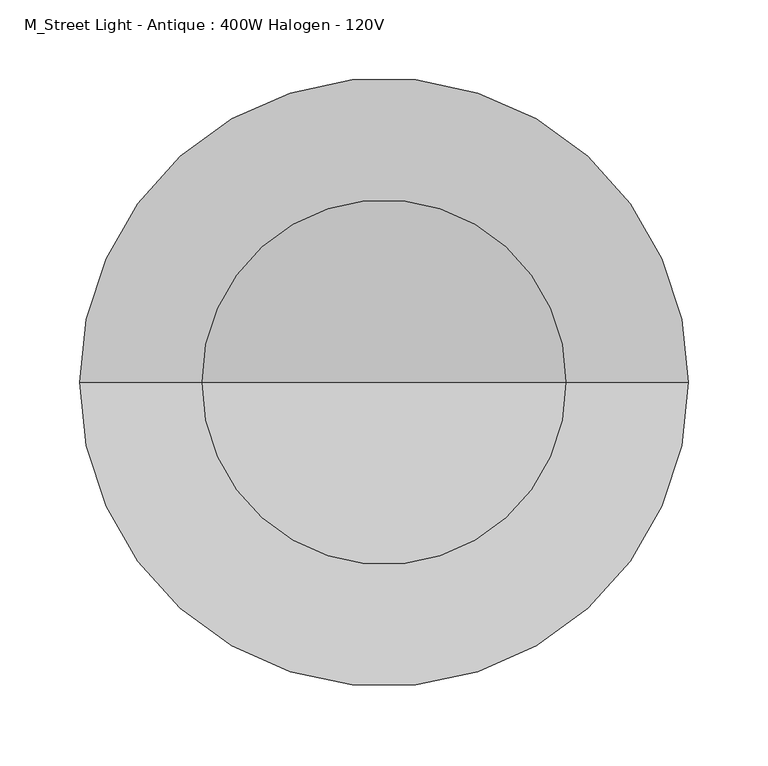
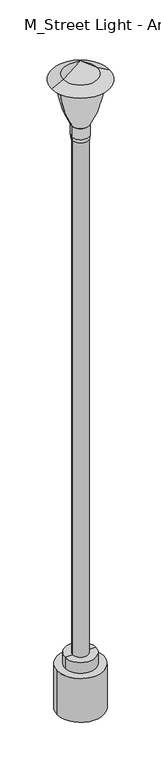
"""IFC4 building model written with IfcOpenShell, lengths in millimetres: light fixture geometry, M_Street Light - Antique : 400W Halogen - 120V."""

from ifc_helpers import new_model, si_unit, point, frame, origin, origin_with_axes, origin_2d, place, context, project, spatial, polyline, circle_curve, ellipse_curve, trimmed, segment, composite_curve, outline, extrude, source, transform, mapped, element, save
from ifc_brep_helpers import plane_surface, cylinder_surface, revolved_surface, advanced_brep


def m_street_light_antique_400w_halogen_120v_ac89fb25(model_context):
    return source(origin(), model_context, "Body", "SolidModel", [
        extrude(outline(composite_curve([segment(trimmed(circle_curve(origin_2d(), 152.4), [point((-152.4, 0.0))], [point((152.4, 0.0))], False, "CARTESIAN"), True, "CONTINUOUS"), segment(trimmed(circle_curve(origin_2d(), 152.4), [point((152.4, 0.0))], [point((-152.4, 0.0))], False, "CARTESIAN"), True, "CONTINUOUS")], self_intersect=False)), origin_with_axes(), (0.0, 0.0, 1.0), 304.8),
        advanced_brep(
        [(190.5, 0.0, 4373.0), (-190.5, 0.0, 4373.0), (-114.3, 0.0, 4411.1), (114.3, 0.0, 4411.1), (114.3, 0.0, 4373.0), (-114.3, 0.0, 4373.0), (114.3, 0.0, 4381.73125), (-114.3, 0.0, 4381.73125), (144.6394367, 0.0, 4381.73125), (-144.6394367, 0.0, 4381.73125), (107.4535144, 0.0, 4400.3242111), (-107.4535144, 0.0, 4400.3242111), (0.0, 0.0, 4485.1715369), (0.0, 0.0, 4500.0)],
        [
            (0, 1, circle_curve(frame((0.0, 0.0, 4373.0), z_axis=(0.0, 0.0, 1.0), x_axis=(-1.0, 0.0, 0.0)), 190.5)),
            (1, 2),
            (2, 3, circle_curve(frame((0.0, 0.0, 4411.1), z_axis=(0.0, 0.0, -1.0), x_axis=(-1.0, 0.0, 0.0)), 114.3)),
            (3, 0),
            (1, 0, circle_curve(frame((0.0, 0.0, 4373.0), z_axis=(0.0, 0.0, 1.0), x_axis=(-1.0, 0.0, 0.0)), 190.5)),
            (3, 2, circle_curve(frame((0.0, 0.0, 4411.1), z_axis=(0.0, 0.0, -1.0), x_axis=(-1.0, 0.0, 0.0)), 114.3)),
            (4, 5, circle_curve(frame((0.0, 0.0, 4373.0), z_axis=(0.0, 0.0, 1.0), x_axis=(-1.0, 0.0, 0.0)), 114.3)),
            (5, 1),
            (0, 4),
            (5, 4, circle_curve(frame((0.0, 0.0, 4373.0), z_axis=(0.0, 0.0, 1.0), x_axis=(-1.0, 0.0, 0.0)), 114.3)),
            (6, 7, circle_curve(frame((0.0, 0.0, 4381.73125), z_axis=(0.0, 0.0, 1.0), x_axis=(-1.0, 0.0, 0.0)), 114.3)),
            (7, 5),
            (4, 6),
            (7, 6, circle_curve(frame((0.0, 0.0, 4381.73125), z_axis=(0.0, 0.0, 1.0), x_axis=(-1.0, 0.0, 0.0)), 114.3)),
            (8, 9, circle_curve(frame((0.0, 0.0, 4381.73125), z_axis=(0.0, 0.0, 1.0), x_axis=(-1.0, 0.0, 0.0)), 144.6394367)),
            (9, 7),
            (6, 8),
            (9, 8, circle_curve(frame((0.0, 0.0, 4381.73125), z_axis=(0.0, 0.0, 1.0), x_axis=(-1.0, 0.0, 0.0)), 144.6394367)),
            (10, 11, circle_curve(frame((0.0, 0.0, 4400.3242111), z_axis=(0.0, 0.0, 1.0), x_axis=(-1.0, 0.0, 0.0)), 107.4535144)),
            (11, 9),
            (8, 10),
            (11, 10, circle_curve(frame((0.0, 0.0, 4400.3242111), z_axis=(0.0, 0.0, 1.0), x_axis=(-1.0, 0.0, 0.0)), 107.4535144)),
            (12, 11),
            (10, 12),
            (2, 13),
            (13, 3),
        ],
        [
            revolved_surface(polyline([(-114.3, 0.0, 4411.1), (-190.5, 0.0, 4373.0)]), (0.0, 0.0, 4754.0), (0.0, 0.0, -1.0)),
            plane_surface(frame((0.0, 0.0, 4373.0), z_axis=(0.0, 0.0, -1.0), x_axis=(-1.0, 0.0, 0.0))),
            revolved_surface(polyline([(-114.3, 0.0, 4373.0), (-114.3, 0.0, 4381.73125)]), (0.0, 0.0, 4754.0), (0.0, 0.0, -1.0)),
            plane_surface(frame((0.0, 0.0, 4381.73125), z_axis=(0.0, 0.0, 1.0), x_axis=(-1.0, 0.0, 0.0))),
            revolved_surface(polyline([(-144.6394367, 0.0, 4381.73125), (-107.4535144, 0.0, 4400.3242111)]), (0.0, 0.0, 4754.0), (0.0, 0.0, -1.0)),
            revolved_surface(polyline([(-107.4535144, 0.0, 4400.3242111), (0.0, 0.0, 4485.1715369)]), (0.0, 0.0, 4754.0), (0.0, 0.0, -1.0)),
            revolved_surface(polyline([(0.0, 0.0, 4500.0), (-114.3, 0.0, 4411.1)]), (0.0, 0.0, 4754.0), (0.0, 0.0, -1.0)),
        ],
        [
            (0, [[1, 2, 3, 4]]),
            (0, [[5, -4, 6, -2]]),
            (1, [[7, 8, -1, 9]]),
            (1, [[10, -9, -5, -8]]),
            (2, [[11, 12, -7, 13]]),
            (2, [[14, -13, -10, -12]]),
            (3, [[15, 16, -11, 17]]),
            (3, [[18, -17, -14, -16]]),
            (4, [[19, 20, -15, 21]]),
            (4, [[22, -21, -18, -20]]),
            (5, [[23, -19, 24]]),
            (5, [[-24, -22, -23]]),
            (6, [[-3, 25, 26]]),
            (6, [[-6, -26, -25]]),
        ],
    ),
        advanced_brep(
        [(53.975, 0.0, 3992.0), (-53.975, 0.0, 3992.0), (-57.3982763, 0.0, 3992.0), (57.3982763, 0.0, 3992.0), (53.975, 0.0, 3966.6), (-53.975, 0.0, 3966.6), (12.7, 0.0, 3966.6), (-12.7, 0.0, 3966.6), (12.7, 0.0, 3992.0), (-12.7, 0.0, 3992.0), (31.9982763, 0.0, 3992.0), (-31.9982763, 0.0, 3992.0), (31.9982763, 0.0, 4068.2), (-31.9982763, 0.0, 4068.2), (57.3982763, 0.0, 4068.2), (-57.3982763, 0.0, 4068.2)],
        [
            (0, 1, circle_curve(frame((0.0, 0.0, 3992.0), z_axis=(0.0, 0.0, 1.0), x_axis=(-1.0, 0.0, 0.0)), 53.975)),
            (1, 2),
            (2, 3, circle_curve(frame((0.0, 0.0, 3992.0), z_axis=(0.0, 0.0, -1.0), x_axis=(-1.0, 0.0, 0.0)), 57.3982763)),
            (3, 0),
            (1, 0, circle_curve(frame((0.0, 0.0, 3992.0), z_axis=(0.0, 0.0, 1.0), x_axis=(-1.0, 0.0, 0.0)), 53.975)),
            (3, 2, circle_curve(frame((0.0, 0.0, 3992.0), z_axis=(0.0, 0.0, -1.0), x_axis=(-1.0, 0.0, 0.0)), 57.3982763)),
            (4, 5, circle_curve(frame((0.0, 0.0, 3966.6), z_axis=(0.0, 0.0, 1.0), x_axis=(-1.0, 0.0, 0.0)), 53.975)),
            (5, 1),
            (0, 4),
            (5, 4, circle_curve(frame((0.0, 0.0, 3966.6), z_axis=(0.0, 0.0, 1.0), x_axis=(-1.0, 0.0, 0.0)), 53.975)),
            (6, 7, circle_curve(frame((0.0, 0.0, 3966.6), z_axis=(0.0, 0.0, 1.0), x_axis=(-1.0, 0.0, 0.0)), 12.7)),
            (7, 5),
            (4, 6),
            (7, 6, circle_curve(frame((0.0, 0.0, 3966.6), z_axis=(0.0, 0.0, 1.0), x_axis=(-1.0, 0.0, 0.0)), 12.7)),
            (8, 9, circle_curve(frame((0.0, 0.0, 3992.0), z_axis=(0.0, 0.0, 1.0), x_axis=(-1.0, 0.0, 0.0)), 12.7)),
            (9, 7),
            (6, 8),
            (9, 8, circle_curve(frame((0.0, 0.0, 3992.0), z_axis=(0.0, 0.0, 1.0), x_axis=(-1.0, 0.0, 0.0)), 12.7)),
            (10, 11, circle_curve(frame((0.0, 0.0, 3992.0), z_axis=(0.0, 0.0, 1.0), x_axis=(-1.0, 0.0, 0.0)), 31.9982763)),
            (11, 9),
            (8, 10),
            (11, 10, circle_curve(frame((0.0, 0.0, 3992.0), z_axis=(0.0, 0.0, 1.0), x_axis=(-1.0, 0.0, 0.0)), 31.9982763)),
            (12, 13, circle_curve(frame((0.0, 0.0, 4068.2), z_axis=(0.0, 0.0, 1.0), x_axis=(-1.0, 0.0, 0.0)), 31.9982763)),
            (13, 11),
            (10, 12),
            (13, 12, circle_curve(frame((0.0, 0.0, 4068.2), z_axis=(0.0, 0.0, 1.0), x_axis=(-1.0, 0.0, 0.0)), 31.9982763)),
            (14, 15, circle_curve(frame((0.0, 0.0, 4068.2), z_axis=(0.0, 0.0, 1.0), x_axis=(-1.0, 0.0, 0.0)), 57.3982763)),
            (15, 13),
            (12, 14),
            (15, 14, circle_curve(frame((0.0, 0.0, 4068.2), z_axis=(0.0, 0.0, 1.0), x_axis=(-1.0, 0.0, 0.0)), 57.3982763)),
            (2, 15),
            (14, 3),
        ],
        [
            plane_surface(frame((0.0, 0.0, 3992.0), z_axis=(0.0, 0.0, -1.0), x_axis=(-1.0, 0.0, 0.0))),
            cylinder_surface(frame((0.0, 0.0, 4754.0), z_axis=(0.0, 0.0, -1.0), x_axis=(-1.0, 0.0, 0.0)), 53.975),
            plane_surface(frame((0.0, 0.0, 3966.6), z_axis=(0.0, 0.0, -1.0), x_axis=(-1.0, 0.0, 0.0))),
            revolved_surface(polyline([(-12.7, 0.0, 3966.6), (-12.7, 0.0, 3992.0)]), (0.0, 0.0, 4754.0), (0.0, 0.0, -1.0)),
            plane_surface(frame((0.0, 0.0, 3992.0), z_axis=(0.0, 0.0, 1.0), x_axis=(-1.0, 0.0, 0.0))),
            revolved_surface(polyline([(-31.9982763, 0.0, 3992.0), (-31.9982763, 0.0, 4068.2)]), (0.0, 0.0, 4754.0), (0.0, 0.0, -1.0)),
            plane_surface(frame((0.0, 0.0, 4068.2), z_axis=(0.0, 0.0, 1.0), x_axis=(-1.0, 0.0, 0.0))),
            cylinder_surface(frame((0.0, 0.0, 4754.0), z_axis=(0.0, 0.0, -1.0), x_axis=(-1.0, 0.0, 0.0)), 57.3982763),
        ],
        [
            (0, [[1, 2, 3, 4]]),
            (0, [[5, -4, 6, -2]]),
            (1, [[7, 8, -1, 9]]),
            (1, [[10, -9, -5, -8]]),
            (2, [[11, 12, -7, 13]]),
            (2, [[14, -13, -10, -12]]),
            (3, [[15, 16, -11, 17]]),
            (3, [[18, -17, -14, -16]]),
            (4, [[19, 20, -15, 21]]),
            (4, [[22, -21, -18, -20]]),
            (5, [[23, 24, -19, 25]]),
            (5, [[26, -25, -22, -24]]),
            (6, [[27, 28, -23, 29]]),
            (6, [[30, -29, -26, -28]]),
            (7, [[-3, 31, -27, 32]]),
            (7, [[-6, -32, -30, -31]]),
        ],
    ),
        advanced_brep(
        [(101.6, 0.0, 381.0), (-101.6, 0.0, 381.0), (-101.6, 0.0, 304.8), (101.6, 0.0, 304.8), (50.8, 0.0, 381.0), (-50.8, 0.0, 381.0), (50.8, 0.0, 3966.6), (-50.8, 0.0, 3966.6), (25.4, 0.0, 3966.6), (-25.4, 0.0, 3966.6), (25.4, 0.0, 304.8), (-25.4, 0.0, 304.8)],
        [
            (0, 1, circle_curve(frame((0.0, 0.0, 381.0), z_axis=(0.0, 0.0, -1.0), x_axis=(-1.0, 0.0, 0.0)), 101.6)),
            (1, 2),
            (2, 3, circle_curve(frame((0.0, 0.0, 304.8), z_axis=(0.0, 0.0, 1.0), x_axis=(-1.0, 0.0, 0.0)), 101.6)),
            (3, 0),
            (4, 5, circle_curve(frame((0.0, 0.0, 381.0), z_axis=(0.0, 0.0, -1.0), x_axis=(-1.0, 0.0, 0.0)), 50.8)),
            (5, 1),
            (0, 4),
            (6, 7, circle_curve(frame((0.0, 0.0, 3966.6), z_axis=(0.0, 0.0, -1.0), x_axis=(-1.0, 0.0, 0.0)), 50.8)),
            (7, 5),
            (4, 6),
            (8, 9, circle_curve(frame((0.0, 0.0, 3966.6), z_axis=(0.0, 0.0, -1.0), x_axis=(-1.0, 0.0, 0.0)), 25.4)),
            (9, 7),
            (6, 8),
            (10, 11, circle_curve(frame((0.0, 0.0, 304.8), z_axis=(0.0, 0.0, -1.0), x_axis=(-1.0, 0.0, 0.0)), 25.4)),
            (11, 9),
            (8, 10),
            (2, 11),
            (10, 3),
            (1, 0, circle_curve(frame((0.0, 0.0, 381.0), z_axis=(0.0, 0.0, -1.0), x_axis=(1.0, 0.0, 0.0)), 101.6)),
            (3, 2, circle_curve(frame((0.0, 0.0, 304.8), z_axis=(0.0, 0.0, 1.0), x_axis=(1.0, 0.0, 0.0)), 101.6)),
            (5, 4, circle_curve(frame((0.0, 0.0, 381.0), z_axis=(0.0, 0.0, -1.0), x_axis=(1.0, 0.0, 0.0)), 50.8)),
            (7, 6, circle_curve(frame((0.0, 0.0, 3966.6), z_axis=(0.0, 0.0, -1.0), x_axis=(1.0, 0.0, 0.0)), 50.8)),
            (9, 8, circle_curve(frame((0.0, 0.0, 3966.6), z_axis=(0.0, 0.0, -1.0), x_axis=(1.0, 0.0, 0.0)), 25.4)),
            (11, 10, circle_curve(frame((0.0, 0.0, 304.8), z_axis=(0.0, 0.0, -1.0), x_axis=(1.0, 0.0, 0.0)), 25.4)),
        ],
        [
            cylinder_surface(frame((0.0, 0.0, 304.8), z_axis=(0.0, 0.0, 1.0), x_axis=(-1.0, 0.0, 0.0)), 101.6),
            plane_surface(frame((0.0, 0.0, 381.0), z_axis=(0.0, 0.0, 1.0), x_axis=(-1.0, 0.0, 0.0))),
            cylinder_surface(frame((0.0, 0.0, 304.8), z_axis=(0.0, 0.0, 1.0), x_axis=(-1.0, 0.0, 0.0)), 50.8),
            plane_surface(frame((0.0, 0.0, 3966.6), z_axis=(0.0, 0.0, 1.0), x_axis=(-1.0, 0.0, 0.0))),
            revolved_surface(polyline([(-25.4, 0.0, 3966.6), (-25.4, 0.0, 304.8)]), (0.0, 0.0, 304.8), (0.0, 0.0, 1.0)),
            plane_surface(frame((0.0, 0.0, 304.8), z_axis=(0.0, 0.0, -1.0), x_axis=(-1.0, 0.0, 0.0))),
            cylinder_surface(frame((0.0, 0.0, 304.8), z_axis=(0.0, 0.0, 1.0), x_axis=(1.0, 0.0, 0.0)), 101.6),
            plane_surface(frame((0.0, 0.0, 381.0), z_axis=(0.0, 0.0, 1.0), x_axis=(1.0, 0.0, 0.0))),
            cylinder_surface(frame((0.0, 0.0, 304.8), z_axis=(0.0, 0.0, 1.0), x_axis=(1.0, 0.0, 0.0)), 50.8),
            plane_surface(frame((0.0, 0.0, 3966.6), z_axis=(0.0, 0.0, 1.0), x_axis=(1.0, 0.0, 0.0))),
            revolved_surface(polyline([(25.4, 0.0, 3966.6), (25.4, 0.0, 304.8)]), (0.0, 0.0, 304.8), (0.0, 0.0, 1.0)),
            plane_surface(frame((0.0, 0.0, 304.8), z_axis=(0.0, 0.0, -1.0), x_axis=(1.0, 0.0, 0.0))),
        ],
        [
            (0, [[1, 2, 3, 4]]),
            (1, [[5, 6, -1, 7]]),
            (2, [[8, 9, -5, 10]]),
            (3, [[11, 12, -8, 13]]),
            (4, [[14, 15, -11, 16]]),
            (5, [[-3, 17, -14, 18]]),
            (6, [[19, -4, 20, -2]]),
            (7, [[21, -7, -19, -6]]),
            (8, [[22, -10, -21, -9]]),
            (9, [[23, -13, -22, -12]]),
            (10, [[24, -16, -23, -15]]),
            (11, [[-20, -18, -24, -17]]),
        ],
    ),
        advanced_brep(
        [(57.3982763, 0.0, 4068.2), (-57.3982763, 0.0, 4068.2), (-139.0691901, 0.0, 4373.0), (139.0691901, 0.0, 4373.0), (51.0432576, 0.0, 4068.2), (-51.0432576, 0.0, 4068.2), (131.8784122, 0.0, 4373.0), (-131.8784122, 0.0, 4373.0)],
        [
            (0, 1, circle_curve(frame((0.0, 0.0, 4068.2), z_axis=(0.0, 0.0, 1.0), x_axis=(-1.0, 0.0, 0.0)), 57.3982763)),
            (1, 2, circle_curve(frame((555.9362168, 0.0, 4395.8843098), z_axis=(0.0, 1.0, 0.0), x_axis=(1.0, 0.0, 0.0)), 695.3820586)),
            (2, 3, circle_curve(frame((0.0, 0.0, 4373.0), z_axis=(0.0, 0.0, -1.0), x_axis=(-1.0, 0.0, 0.0)), 139.0691901)),
            (3, 0, circle_curve(frame((-555.9362168, 0.0, 4395.8843098), z_axis=(0.0, 1.0, 0.0), x_axis=(-1.0, 0.0, 0.0)), 695.3820586)),
            (1, 0, circle_curve(frame((0.0, 0.0, 4068.2), z_axis=(0.0, 0.0, 1.0), x_axis=(-1.0, 0.0, 0.0)), 57.3982763)),
            (3, 2, circle_curve(frame((0.0, 0.0, 4373.0), z_axis=(0.0, 0.0, -1.0), x_axis=(-1.0, 0.0, 0.0)), 139.0691901)),
            (4, 5, circle_curve(frame((0.0, 0.0, 4068.2), z_axis=(0.0, 0.0, 1.0), x_axis=(-1.0, 0.0, 0.0)), 51.0432576)),
            (5, 1),
            (0, 4),
            (5, 4, circle_curve(frame((0.0, 0.0, 4068.2), z_axis=(0.0, 0.0, 1.0), x_axis=(-1.0, 0.0, 0.0)), 51.0432576)),
            (6, 7, circle_curve(frame((0.0, 0.0, 4373.0), z_axis=(0.0, 0.0, 1.0), x_axis=(-1.0, 0.0, 0.0)), 131.8784122)),
            (7, 5, circle_curve(frame((563.1799394, 0.0, 4394.2154469), z_axis=(0.0, -1.0, 0.0), x_axis=(1.0, 0.0, 0.0)), 695.3820586)),
            (4, 6, circle_curve(frame((-563.1799394, 0.0, 4394.2154469), z_axis=(0.0, -1.0, 0.0), x_axis=(-1.0, 0.0, 0.0)), 695.3820586)),
            (7, 6, circle_curve(frame((0.0, 0.0, 4373.0), z_axis=(0.0, 0.0, 1.0), x_axis=(-1.0, 0.0, 0.0)), 131.8784122)),
            (2, 7),
            (6, 3),
        ],
        [
            revolved_surface(trimmed(ellipse_curve(frame((555.9362168, 0.0, 4395.8843098), z_axis=(0.0, -1.0, 0.0), x_axis=(1.0, 0.0, 0.0)), 695.3820586, 695.3820586), [point((-139.0691901, 0.0, 4373.0))], [point((-57.3982763, 0.0, 4068.2))], True, "CARTESIAN"), (0.0, 0.0, 4677.8), (0.0, 0.0, -1.0)),
            plane_surface(frame((0.0, 0.0, 4068.2), z_axis=(0.0, 0.0, -1.0), x_axis=(-1.0, 0.0, 0.0))),
            revolved_surface(trimmed(ellipse_curve(frame((563.1799394, 0.0, 4394.2154469), z_axis=(0.0, 1.0, 0.0), x_axis=(1.0, 0.0, 0.0)), 695.3820586, 695.3820586), [point((-51.0432576, 0.0, 4068.2))], [point((-131.8784122, 0.0, 4373.0))], True, "CARTESIAN"), (0.0, 0.0, 4677.8), (0.0, 0.0, -1.0)),
            plane_surface(frame((0.0, 0.0, 4373.0), z_axis=(0.0, 0.0, 1.0), x_axis=(-1.0, 0.0, 0.0))),
        ],
        [
            (0, [[1, 2, 3, 4]]),
            (0, [[5, -4, 6, -2]]),
            (1, [[7, 8, -1, 9]]),
            (1, [[10, -9, -5, -8]]),
            (2, [[11, 12, -7, 13]]),
            (2, [[14, -13, -10, -12]]),
            (3, [[-3, 15, -11, 16]]),
            (3, [[-6, -16, -14, -15]]),
        ],
    ),
    ])


if __name__ == "__main__":
    model = new_model("IFC4")
    model_context = context("Model", 3, world=origin())
    ifc_project = project(units=[si_unit("LENGTHUNIT", "METRE", prefix="MILLI")], contexts=[model_context])
    site = spatial("IfcSite", under=ifc_project)
    building = spatial("IfcBuilding", under=site)
    placement = place(None, origin())
    m_street_light_antique_400w_halogen_120v_shape = m_street_light_antique_400w_halogen_120v_ac89fb25(model_context)
    element("IfcLightFixture", 1, ObjectType="M_Street Light - Antique : 400W Halogen - 120V", at=placement, inside=building, context=model_context, shape_type="MappedRepresentation", body=[
        mapped(m_street_light_antique_400w_halogen_120v_shape, transform((0.0, 0.0, 0.0), x_axis=(1.0, 0.0, 0.0), y_axis=(0.0, 1.0, 0.0), z_axis=(0.0, 0.0, 1.0))),
    ])
    save(model, "model.ifc")

# Revit data of these elements
# Type "M_Street Light - Antique : 400W Halogen - 120V"
#   Photometric Web File = "SLS1T3.ies"
#   Assembly Code = "D5020280"
#   Lamp = "T-3"
#   Wattage Comments = "400"
#   Wattage = 1000 W
#   built-in parameter 1150110 = 2 (stored number, unit not read)
#   built-in parameter 1114217 = 4 (stored number, unit not read)
#   built-in parameter 1150109 = 2 (stored number, unit not read)
#   built-in parameter 1150113 = 1 (stored number, unit not read)
#   Tilt Angle = -90.00°
#   built-in parameter 1150115 = 1 (stored number, unit not read)
#   built-in parameter 1150105 = 7957.75 (stored number, unit not read)
#   built-in parameter 1150112 = 1 (stored number, unit not read)
#   built-in parameter 1150114 = 1 (stored number, unit not read)
#   built-in parameter 1150107 = 8000 (stored number, unit not read)
#   built-in parameter 1150106 = 79.5775 (stored number, unit not read)
#   built-in parameter 1150104 = 9.2903 (stored number, unit not read)
#   Voltage = 120 V
#   built-in parameter 1114218 = 1 (stored number, unit not read)
#   built-in parameter 1150133 = 10 (stored number, unit not read)
#   Height = 14' - 9.16535"
#   Lumens = 100000 lm
#   Apparent Load = 400 VA
#   built-in parameter 1150137 = 1
#   Color Filter = 16777215
#   Number of poles = 1
#   Shade Material = none
#   Load Classification = Lighting - Exterior
#   Diffuser Material = Glass, Frosted
#   Stand Material = Steel, Paint Finish, Dark Gray, Matte
#   Dimming Lamp Color Temperature Shift = (empty or 0)
#   Default Elevation = 0
# Element 1 (IfcLightFixture, "M_Street Light - Antique : 400W Halogen - 120V")
#   Materials on its faces: "Steel, Paint Finish, Dark Gray, Matte", "Glass, Frosted"
# Materials
#   "Glass, Frosted": class "Glass", colour RGB 249 250 249, transparency 0.8, Description = "physical material", Cost = 0
#   "Steel, Paint Finish, Dark Gray, Matte": class "Metal", colour RGB 98 98 98, transparency 0, Description = "Steel, paint finish, dark gray, matte", Cost = 0
